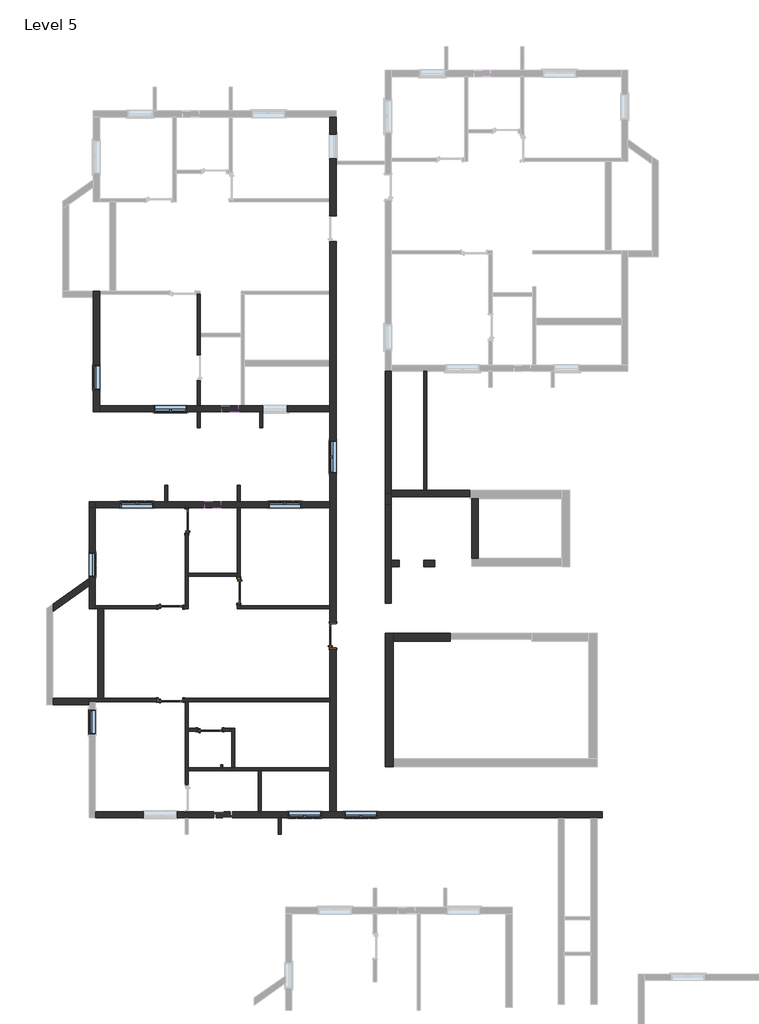
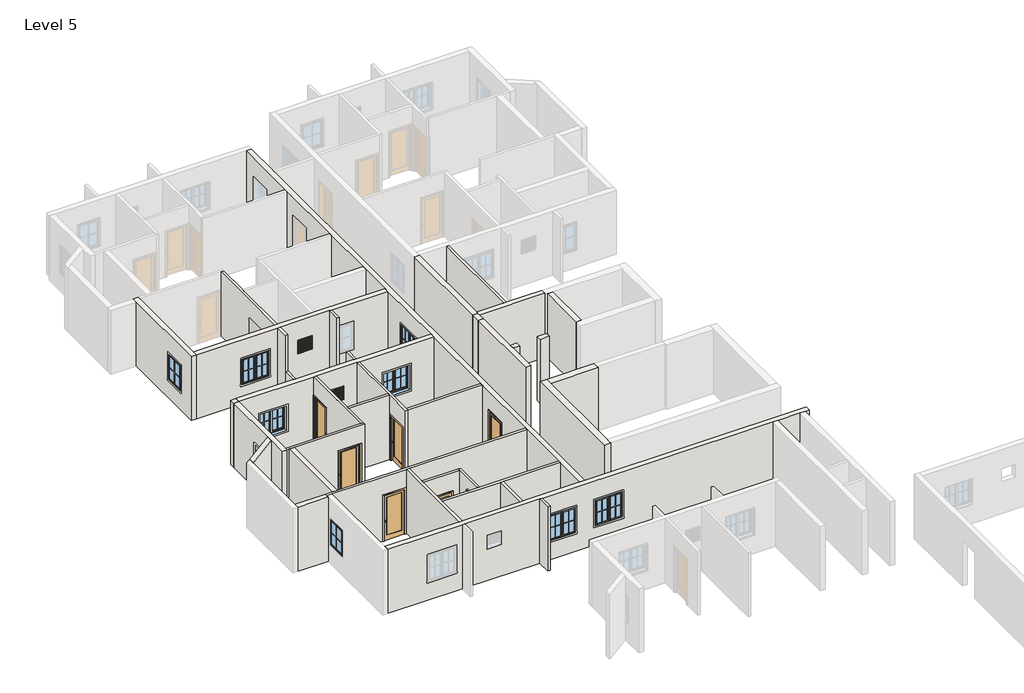
# One storey, part 4 of 7: 38 walls, 11 windows, 6 doors.
# Revit data of these elements (continued)
# Element 46 (IfcWindow, "Window-Awning-Single : 36\" x 48\"") (continued)
#   Mark = "87"
#   Window Inset = 0' - 0"
#   Interior Wall Closure = 0' - 2 1/4"
#   Frame Extension = 0' - 0 1/4"
#   Exterior Wall Closure = 0' - 1 1/4"
#   Interior Trim Visibility = yes
#   Exterior Trim Visibility = yes
#   Phase Created = New Construction
#   Materials on its faces: "Wood - Stained", "Glass", "Clad - White"
# Element 47 (IfcWindow, "Window-Awning-Single : 36\" x 48\"")
#   Mark = "99"
#   Window Inset = 0' - 0"
#   Interior Wall Closure = 0' - 2 1/4"
#   Frame Extension = 0' - 0 1/4"
#   Exterior Wall Closure = 0' - 1 1/4"
#   Interior Trim Visibility = yes
#   Exterior Trim Visibility = yes
#   Phase Created = New Construction
#   Materials on its faces: "Wood - Stained", "Glass", "Clad - White"
# Element 48 (IfcWindow, "Window-Casement-Double : 4' x 4'")
#   Mark = "102"
#   Window Inset = 0' - 0"
#   Interior Wall Closure = 0' - 2 1/4"
#   Frame Extension = 0' - 0 1/4"
#   Exterior Wall Closure = 0' - 1 1/4"
#   Interior Trim Visibility = yes
#   Exterior Trim Visibility = yes
#   Phase Created = New Construction
#   Materials on its faces: "Wood - Stained", "Glass", "Clad - White"
# Element 49 (IfcWindow, "Window-Casement-Double : 4' x 4'")
#   Mark = "127"
#   Window Inset = 0' - 0"
#   Interior Wall Closure = 0' - 2 1/4"
#   Frame Extension = 0' - 0 1/4"
#   Exterior Wall Closure = 0' - 1 1/4"
#   Interior Trim Visibility = yes
#   Exterior Trim Visibility = yes
#   Phase Created = New Construction
#   Materials on its faces: "Wood - Stained", "Glass", "Clad - White"
# Element 50 (IfcWindow, "Window-Casement-Double : 4' x 4'")
#   Mark = "128"
#   Window Inset = 0' - 0"
#   Interior Wall Closure = 0' - 2 1/4"
#   Frame Extension = 0' - 0 1/4"
#   Exterior Wall Closure = 0' - 1 1/4"
#   Interior Trim Visibility = yes
#   Exterior Trim Visibility = yes
#   Phase Created = New Construction
#   Materials on its faces: "Wood - Stained", "Glass", "Clad - White"
# Element 51 (IfcWindow, "Window-Casement-Double : 4' x 4'")
#   Mark = "130"
#   Window Inset = 0' - 0"
#   Interior Wall Closure = 0' - 2 1/4"
#   Frame Extension = 0' - 0 1/4"
#   Exterior Wall Closure = 0' - 1 1/4"
#   Interior Trim Visibility = yes
#   Exterior Trim Visibility = yes
#   Phase Created = New Construction
#   Materials on its faces: "Wood - Stained", "Glass", "Clad - White"
# Element 52 (IfcWindow, "Window-Casement-Double : 4' x 4'")
#   Mark = "131"
#   Window Inset = 0' - 0"
#   Interior Wall Closure = 0' - 2 1/4"
#   Frame Extension = 0' - 0 1/4"
#   Exterior Wall Closure = 0' - 1 1/4"
#   Interior Trim Visibility = yes
#   Exterior Trim Visibility = yes
#   Phase Created = New Construction
#   Materials on its faces: "Wood - Stained", "Glass", "Clad - White"
# Element 53 (IfcWindow, "Window-Casement-Double : 4' x 4'")
#   Mark = "132"
#   Window Inset = 0' - 0"
#   Interior Wall Closure = 0' - 2 1/4"
#   Frame Extension = 0' - 0 1/4"
#   Exterior Wall Closure = 0' - 1 1/4"
#   Interior Trim Visibility = yes
#   Exterior Trim Visibility = yes
#   Phase Created = New Construction
#   Materials on its faces: "Wood - Stained", "Glass", "Clad - White"
# Element 54 (IfcWindow, "Window-Louvers : 24\" x 24\"")
#   Mark = "68"
#   Blade Width = 1' - 10 1/2"
#   Phase Created = New Construction
#   Materials on its faces: "Birch"
# Element 55 (IfcWindow, "Window-Louvers : 24\" x 24\"")
#   Mark = "71"
#   Blade Width = 1' - 10 1/2"
#   Phase Created = New Construction
#   Materials on its faces: "Birch"
# Materials
#   "Cherry": class "Wood", colour RGB 226 177 128, transparency 0, Description = "Prunus Serotina", Cost = 0
#   "Aluminum": class "Metal", colour RGB 247 247 247, transparency 0, Description = "Aluminum 6061", Cost = 0
#   "Wood - Stained": class "Wood", colour RGB 224 178 126, transparency 0, Cost = 0
#   "Glass": class "Glass", colour RGB 0 128 192, transparency 0.75, Description = "Soda Lime Glass", Cost = 0
#   "Clad - White": class "Wood", colour RGB 242 242 238, transparency 0, Cost = 0
#   "Birch": class "Wood", colour RGB 224 178 126, transparency 0, Description = "Betula Alleghaniensis", Cost = 0
#   "Default Wall": colour RGB 128 128 128, transparency 0, Cost = 0
